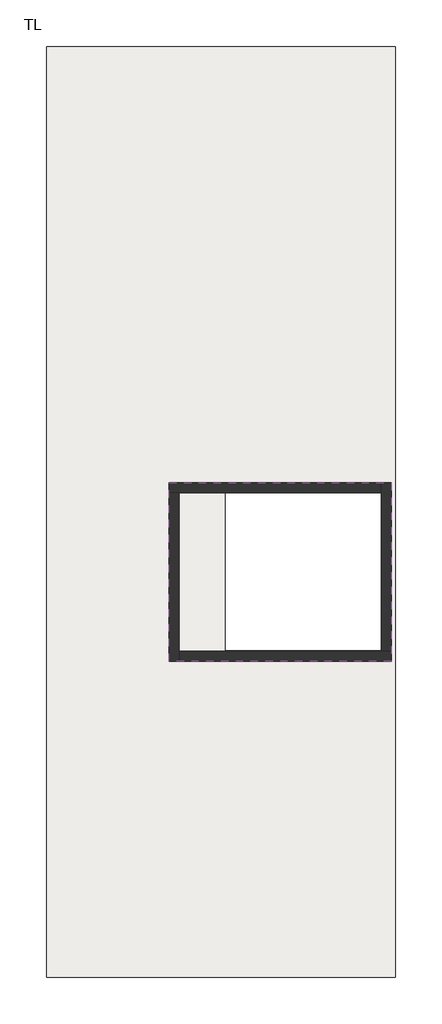
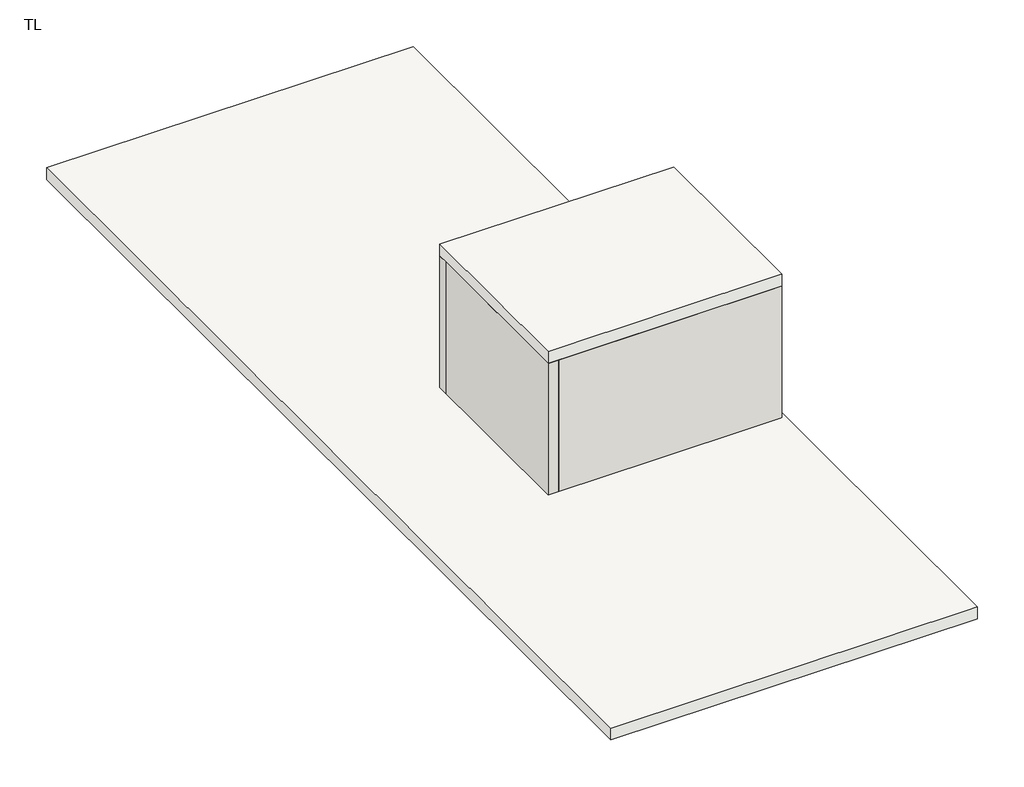
# One storey: 4 walls, 2 slabs.
"""IFC4 building model written with IfcOpenShell, lengths in millimetres."""

from ifc_helpers import new_model, si_unit, frame, origin, place, context, project, spatial, polyline, outline, extrude, faceted_brep, element, save

model = new_model("IFC4")

# Units and contexts
model_context = context("Model", 3, world=origin())
ifc_project = project(units=[si_unit("LENGTHUNIT", "METRE", prefix="MILLI")], contexts=[model_context])

# Site, building, storey
site = spatial("IfcSite", under=ifc_project)
building = spatial("IfcBuilding", under=site)
storey = spatial("IfcBuildingStorey", under=building, Name="TL", Elevation=6000.0)

# Slabs
placement = place(None, origin())
element("IfcSlab", 1, ObjectType="SLAB", at=placement, inside=storey, context=model_context, shape_type="SweptSolid", body=[
    extrude(outline(polyline([(-16105.0702358, 13896.3258404), (-16105.0702358, -132.2741596), (-21365.6794706, -132.2741596), (-21365.6794706, 13896.3258404), (-16105.0702358, 13896.3258404)]), holes=[polyline([(-16316.1794706, 7168.7350753), (-18663.7794706, 7168.7350753), (-18663.7794706, 4801.1258404), (-16316.1794706, 4801.1258404), (-16316.1794706, 7168.7350753)])]), frame((0.0, 0.0, 5820.0), z_axis=(0.0, 0.0, 1.0), x_axis=(1.0, 0.0, 0.0)), (0.0, 0.0, 1.0), 180.0),
])
element("IfcSlab", 2, ObjectType="SLAB", at=placement, inside=storey, context=model_context, shape_type="SweptSolid", body=[
    extrude(outline(polyline([(-16163.7794706, 7321.1350753), (-16163.7794706, 4633.5166056), (-19516.1794706, 4633.5166056), (-19516.1794706, 7321.1350753), (-16163.7794706, 7321.1350753)])), frame((0.0, 0.0, 8000.0), z_axis=(0.0, 0.0, 1.0), x_axis=(1.0, 0.0, 0.0)), (0.0, 0.0, 1.0), 180.0),
])

# Walls
element("IfcWall", 3, at=placement, inside=storey, context=model_context, shape_type="Brep", body=[
    faceted_brep([(-19363.7794706, 4633.5166056, 6000.0), (-16163.7794706, 4633.5166056, 6000.0), (-16163.7794706, 4633.5166056, 8000.0), (-19363.7794706, 4633.5166056, 8000.0), (-19363.7794706, 4785.9166056, 6000.0), (-19363.7794706, 4785.9166056, 8000.0), (-16316.1794706, 4785.9166056, 8000.0), (-16163.7794706, 4785.9166056, 8000.0), (-16163.7794706, 4785.9166056, 6000.0), (-16316.1794706, 4785.9166056, 6000.0)], [[[0, 1, 2, 3]], [[4, 5, 6, 7, 8, 9]], [[1, 0, 4, 9, 8]], [[3, 2, 7, 6, 5]], [[2, 1, 8, 7]], [[0, 3, 5, 4]]]),
])
element("IfcWall", 4, at=placement, inside=storey, context=model_context, shape_type="Brep", body=[
    faceted_brep([(-16163.7794706, 4785.9166056, 6000.0), (-16163.7794706, 7321.1350753, 6000.0), (-16163.7794706, 7321.1350753, 8000.0), (-16163.7794706, 4785.9166056, 8000.0), (-16316.1794706, 4785.9166056, 6000.0), (-16316.1794706, 4785.9166056, 8000.0), (-16316.1794706, 7168.7350753, 8000.0), (-16316.1794706, 7321.1350753, 8000.0), (-16316.1794706, 7321.1350753, 6000.0), (-16316.1794706, 7168.7350753, 6000.0)], [[[0, 1, 2, 3]], [[4, 5, 6, 7, 8, 9]], [[1, 0, 4, 9, 8]], [[3, 2, 7, 6, 5]], [[0, 3, 5, 4]], [[2, 1, 8, 7]]]),
])
element("IfcWall", 5, at=placement, inside=storey, context=model_context, shape_type="Brep", body=[
    faceted_brep([(-16316.1794706, 7321.1350753, 6000.0), (-19516.1794706, 7321.1350753, 6000.0), (-19516.1794706, 7321.1350753, 8000.0), (-16316.1794706, 7321.1350753, 8000.0), (-16316.1794706, 7168.7350753, 6000.0), (-16316.1794706, 7168.7350753, 8000.0), (-19363.7794706, 7168.7350753, 8000.0), (-19516.1794706, 7168.7350753, 8000.0), (-19516.1794706, 7168.7350753, 6000.0), (-19363.7794706, 7168.7350753, 6000.0)], [[[0, 1, 2, 3]], [[4, 5, 6, 7, 8, 9]], [[1, 0, 4, 9, 8]], [[3, 2, 7, 6, 5]], [[0, 3, 5, 4]], [[2, 1, 8, 7]]]),
])
element("IfcWall", 6, at=placement, inside=storey, context=model_context, shape_type="Brep", body=[
    faceted_brep([(-19516.1794706, 7168.7350753, 6000.0), (-19516.1794706, 4633.5166056, 6000.0), (-19516.1794706, 4633.5166056, 8000.0), (-19516.1794706, 7168.7350753, 8000.0), (-19363.7794706, 7168.7350753, 6000.0), (-19363.7794706, 7168.7350753, 8000.0), (-19363.7794706, 4785.9166056, 8000.0), (-19363.7794706, 4633.5166056, 8000.0), (-19363.7794706, 4633.5166056, 6000.0), (-19363.7794706, 4785.9166056, 6000.0)], [[[0, 1, 2, 3]], [[4, 5, 6, 7, 8, 9]], [[1, 0, 4, 9, 8]], [[3, 2, 7, 6, 5]], [[0, 3, 5, 4]], [[2, 1, 8, 7]]]),
])

save(model, "model.ifc")

# Revit data of these elements
# Type "SLAB"
#   Layers, outside or top first: 0.18 m "Concrete, Cast In Situ" (function 1)
# Type
#   Keynote = "F10"
#   Layers, outside or top first: 0.1524 m "WHITE BOARD" (function 1)
# Element 1 (IfcSlab, "SLAB")
#   Height Offset From Level = 0.0 m
#   built-in parameter 1001954 = 1
#   Phase Created = New Construction
#   Materials on its faces: "Concrete, Cast In Situ"
# Element 2 (IfcSlab, "SLAB")
#   Height Offset From Level = 2.18 m
#   built-in parameter 1001954 = 1
#   Phase Created = New Construction
#   Materials on its faces: "Concrete, Cast In Situ"
# Elements 3, 4, 5, 6 (IfcWall)
#   Top Offset = 0.0 m
#   Base Offset = 0.0 m
#   Unconnected Height = 2.0 m
#   wall height = 2.0 m
#   Phase Created = New Construction
#   Base Constraint = TL
#   Materials on its faces: "WHITE BOARD"
# Materials
#   "Concrete, Cast In Situ": class "Concrete", colour RGB 192 192 192, transparency 0, Description = "physical material", Cost = 0
#   "WHITE BOARD": class "Generic", colour RGB 249 249 249, transparency 0, Description = "Plaster", Cost = 0
